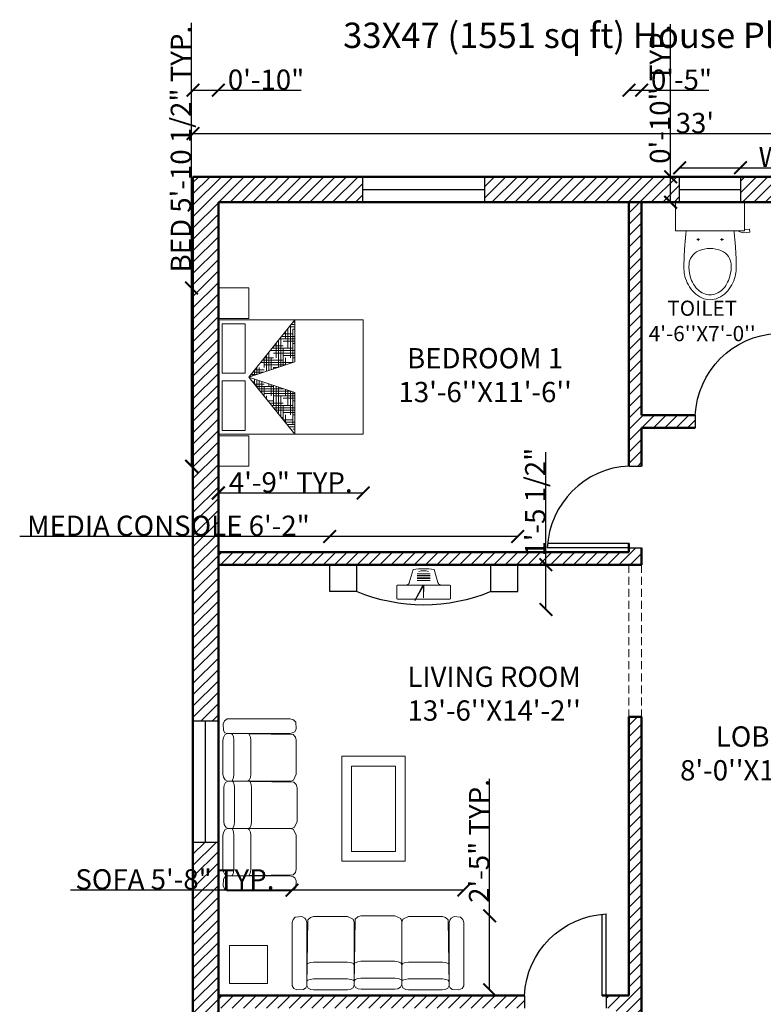
# Model space of a CAD drawing. Units: inches. Extents: x 1875 to 2385, y 1585 to 2263.
# Tile 2 of 3: x 1875 to 2168, y 1875 to 2263. Entities that reach past the tile are written whole.
import ezdxf

# ---------------------------------------------------------------- set-up
doc = ezdxf.new("R2010")
doc.units = ezdxf.units.IN
doc.header["$LTSCALE"] = 0.5
doc.linetypes.add('HIDDEN', pattern=[9.525, 6.35, -3.175])
for name, color, linetype, lineweight in [('A-ANNO-DIMS', 2, 'Continuous', 18), ('A-ANNO-TEXT', 7, 'Continuous', 25), ('A-AREA-IDEN', 7, 'Continuous', 25), ('A-FLOR-FIXT', 9, 'Continuous', 18), ('A-FURN', 8, 'Continuous', 18), ('A-WALL-HIDN', 56, 'HIDDEN', 18), ('A-WALL-PATT', 8, 'Continuous', 13), ('Doors', 42, 'Continuous', 25), ('Walls', 7, 'Continuous', 50), ('Windows', 140, 'Continuous', 25)]:
    doc.layers.add(name, color=color, linetype=linetype, lineweight=lineweight)
doc.layers.add('THIET-BI', color=21, linetype='Continuous')
doc.styles.get("Standard").update_dxf_attribs({"font": 'arial.ttf'})
doc.dimstyles.get("Standard").update_dxf_attribs({"dimtxt": 8, "dimasz": 5, "dimexe": 0.18, "dimexo": 0.0625, "dimgap": 0.09, "dimtad": 1, "dimdec": 1, "dimzin": 0, "dimdsep": 46, "dimlunit": 4, "dimtxsty": 'Standard', "dimblk": 'ARCHTICK', "dimcen": 0.09, "dimse1": 1, "dimse2": 1, "dimadec": 0, "dimazin": 0, "dimtfac": 1, "dimtdec": 1, "dimtofl": 0, "dimtmove": 0, "dimatfit": 3, "dimfxl": 1, "dimtolj": 1, "dimtzin": 0, "dimarcsym": 0})

# ---------------------------------------------------------------- blocks, each defined once
blk = doc.blocks.new('AP0B05')
for p, q in [((35, 100), (35, 880)), ((75, 100), (75, 878.9)), ((35, 100), (35, -20)), ((815, 100), (815, -20))]:
    blk.add_line(p, q)
blk.add_lwpolyline([(35, 100), (75, 100)])
blk.add_arc((-2.4, 62.6), 818.3, 2.62122, 87.37878)
blk = doc.blocks.new('12PCOU17')
at = {"color": 0, "linetype": 'ByBlock'}
for points in [[(-34.71, 34.72), (-33.66, 34.31), (-3.27, 34.3), (-1.81, 34.76), (-1.05, 35.2), (-0.38, 36.65), (-0.61, 39.84), (-1.73, 40.94), (-3.27, 41.4), (-33.66, 41.4), (-34.95, 40.5), (-35.65, 39.02), (-35.49, 35.83), (-34.71, 34.72)], [(-1.89, 11.91), (-1.66, 11.91), (-0.35, 14.68), (-0.35, 31.05), (-0.74, 32.58), (-1.89, 33.83), (-33.63, 34.3), (-34.84, 33.63), (-35.43, 32.38), (-35.68, 31), (-35.68, 14.74), (-35.43, 13.36), (-34.66, 11.99), (-33.44, 11.43), (-3, 11.44), (-1.66, 11.91)], [(-31.25, 11.43), (-31.06, 11.84), (-30.6, 13.09), (-30.4, 14.62), (-30.4, 31.12), (-30.6, 32.65), (-31.06, 33.9), (-31.81, 34.3)], [(-23.84, 11.43), (-22.99, 11.9), (-22.46, 13.15), (-22.23, 14.67), (-22.23, 31.07), (-22.46, 32.59), (-22.99, 33.84), (-23.12, 34.3)], [(-1.54, -10.96), (-1.31, -10.96), (0, -8.19), (0, 8.19), (-0.39, 9.71), (-1.54, 10.96), (-33.28, 11.44), (-34.5, 10.77), (-35.08, 9.51), (-35.33, 8.14), (-35.33, -8.13), (-35.08, -9.51), (-34.31, -10.87), (-33.1, -11.44), (-2.65, -11.43), (-1.31, -10.96)], [(-30.9, -11.44), (-30.72, -11.02), (-30.25, -9.77), (-30.05, -8.25), (-30.05, 8.26), (-30.25, 9.78), (-30.72, 11.03), (-31.47, 11.44)], [(-23.49, -11.44), (-22.64, -10.96), (-22.11, -9.72), (-21.88, -8.19), (-21.88, 8.2), (-22.11, 9.73), (-22.64, 10.97), (-22.77, 11.44)], [(-1.89, -11.91), (-1.66, -11.91), (-0.35, -14.68), (-0.35, -31.05), (-0.74, -32.58), (-1.89, -33.83), (-33.63, -34.3), (-34.84, -33.63), (-35.43, -32.38), (-35.68, -31), (-35.68, -14.74), (-35.43, -13.36), (-34.66, -11.99), (-33.44, -11.43), (-3, -11.44), (-1.66, -11.91)], [(-31.25, -11.43), (-31.06, -11.84), (-30.6, -13.09), (-30.4, -14.62), (-30.4, -31.12), (-30.6, -32.65), (-31.06, -33.9), (-31.81, -34.3)], [(-23.84, -11.43), (-22.99, -11.9), (-22.46, -13.15), (-22.23, -14.67), (-22.23, -31.07), (-22.46, -32.59), (-22.99, -33.84), (-23.12, -34.3)], [(-34.71, -34.72), (-33.66, -34.31), (-3.27, -34.3), (-1.81, -34.76), (-1.05, -35.2), (-0.38, -36.65), (-0.61, -39.84), (-1.73, -40.94), (-3.27, -41.4), (-33.66, -41.4), (-34.95, -40.5), (-35.65, -39.02), (-35.49, -35.83), (-34.71, -34.72)]]:
    blk.add_lwpolyline(points, dxfattribs=at)
blk = doc.blocks.new('*X4')
at = {"color": 0}
for p, q in [((20.174, 14.75), (20.277, 14.75)), ((20.188, 14.75), (20.188, 14.767)), ((20.199, 14.781), (20.277, 14.781)), ((20.25, 14.812), (20.277, 14.812)), ((20.25, 14.319), (20.25, 14.75)), ((20.062, 14.257), (20.062, 14.612)), ((20.094, 14.375), (20.094, 14.65)), ((20.098, 14.656), (20.125, 14.656)), ((20.124, 14.688), (20.25, 14.688)), ((20.125, 14.5), (20.125, 14.689)), ((20.149, 14.719), (20.277, 14.719)), ((20.156, 14.625), (20.156, 14.728)), ((20.219, 14.309), (20.219, 14.625)), ((20.25, 14.625), (20.277, 14.625)), ((19.973, 14.5), (20.25, 14.5)), ((19.998, 14.531), (20.277, 14.531)), ((20, 14.237), (20, 14.5)), ((20.023, 14.562), (20.277, 14.562)), ((20.031, 14.247), (20.031, 14.573)), ((20.125, 14.594), (20.277, 14.594)), ((20.188, 14.299), (20.188, 14.5)), ((19.875, 14.25), (19.875, 14.379)), ((19.875, 14.344), (20.277, 14.344)), ((19.906, 14.375), (19.906, 14.417)), ((19.922, 14.438), (20, 14.438)), ((19.948, 14.469), (20.125, 14.469)), ((19.969, 14.226), (19.969, 14.375)), ((20, 14.375), (20.277, 14.375)), ((20.125, 14.406), (20.277, 14.406)), ((20.156, 14.288), (20.156, 14.375)), ((20.25, 14.438), (20.277, 14.438)), ((19.746, 14.219), (19.875, 14.219)), ((19.75, 14.154), (19.75, 14.223)), ((19.772, 14.25), (20, 14.25)), ((19.781, 14.164), (19.781, 14.262)), ((19.797, 14.281), (20.125, 14.281)), ((19.812, 14.174), (19.812, 14.301)), ((19.822, 14.312), (20.229, 14.312)), ((19.844, 14.185), (19.844, 14.34)), ((19.938, 14.216), (19.938, 14.25)), ((19.702, 14.094), (19.779, 14.094)), ((19.719, 14.073), (19.719, 14.114)), ((19.721, 14.188), (19.75, 14.188)), ((19.75, 14.034), (19.75, 14.103)), ((19.781, 13.995), (19.781, 14.093)), ((19.727, 14.062), (19.873, 14.062)), ((19.752, 14.031), (19.875, 14.031)), ((19.812, 14), (19.812, 14.082)), ((19.875, 13.878), (19.875, 14)), ((19.875, 13.969), (20.156, 13.969)), ((19.906, 13.84), (19.906, 14.051)), ((19.938, 13.801), (19.938, 14.041)), ((19.969, 13.875), (19.969, 14.031)), ((20, 14), (20, 14.02)), ((20, 14), (20.061, 14)), ((20.062, 13.645), (20.062, 14)), ((20.094, 13.625), (20.094, 13.989)), ((20.125, 13.75), (20.125, 13.979)), ((20.156, 13.875), (20.156, 13.969)), ((19.827, 13.938), (20.25, 13.938)), ((19.853, 13.906), (20.125, 13.906)), ((19.878, 13.875), (20, 13.875)), ((20.031, 13.684), (20.031, 13.875)), ((20.125, 13.844), (20.277, 13.844)), ((20.219, 13.451), (20.219, 13.875)), ((20.25, 13.5), (20.25, 13.937)), ((20.25, 13.875), (20.277, 13.875)), ((19.953, 13.781), (20.277, 13.781)), ((19.978, 13.75), (20.25, 13.75)), ((20, 13.812), (20.277, 13.812)), ((20, 13.723), (20, 13.75)), ((20.003, 13.719), (20.125, 13.719)), ((20.188, 13.49), (20.188, 13.75)), ((20.079, 13.625), (20.277, 13.625)), ((20.104, 13.594), (20.277, 13.594)), ((20.125, 13.656), (20.277, 13.656)), ((20.156, 13.529), (20.156, 13.625)), ((20.25, 13.688), (20.277, 13.688)), ((20.129, 13.562), (20.25, 13.562)), ((20.205, 13.469), (20.277, 13.469)), ((20.25, 13.5), (20.277, 13.5)), ((20.23, 13.438), (20.277, 13.438)), ((20.255, 13.406), (20.277, 13.406))]:
    blk.add_line(p, q, dxfattribs=at)
blk = doc.blocks.new('MAT-P13')
for p, q in [((-1.17, 0), (-1.17, -0.4)), ((-1.17, 0), (-0.77, 0)), ((-0.77, 0), (-0.77, -0.4)), ((-0.75, 0), (0.75, 0)), ((-0.75, 0), (-0.75, -1.9)), ((0.75, 0), (0.75, -1.9)), ((0.77, 0), (1.17, 0)), ((0.77, 0), (0.77, -0.4)), ((1.17, 0), (1.17, -0.4)), ((-0.7, -0.05), (-0.7, -0.35)), ((-0.7, -0.05), (-0.05, -0.05)), ((-0.05, -0.35), (-0.05, -0.05)), ((0.05, -0.05), (0.7, -0.05)), ((0.05, -0.35), (0.05, -0.05)), ((0.7, -0.05), (0.7, -0.35)), ((-0.7, -0.35), (-0.05, -0.35)), ((0.05, -0.35), (0.7, -0.35)), ((-1.17, -0.4), (-0.77, -0.4)), ((-0.75, -1.003), (0, -0.4)), ((0, -0.4), (-0.75, -1.003)), ((0, -0.4), (-0.2, -1.003)), ((0, -0.4), (0.2, -1.003)), ((0, -0.4), (0.75, -1.003)), ((0.77, -0.4), (1.17, -0.4)), ((-0.75, -1.003), (-0.2, -1.003)), ((0.2, -1.003), (0.75, -1.003)), ((0.75, -1.9), (-0.75, -1.9))]:
    blk.add_line(p, q)
at = {"xscale": -1, "rotation": 90}
blk.add_blockref('*X4', (14.128, 19.274), dxfattribs=at)
blk = doc.blocks.new('toilet-1')
at = {"color": 0, "linetype": 'ByBlock'}
for p, q in [((-0.23, -0.02), (-0.23, -0.2116)), ((0.23, -0.02), (-0.23, -0.02)), ((0.23, -0.02), (0.23, -0.2116)), ((-0.23, -0.2116), (0.23, -0.2116)), ((-0.0793, -0.2587), (-0.0793, -0.2778)), ((0.0794, -0.2587), (0.0794, -0.2778)), ((0.1917, -0.2144), (0.2206, -0.225)), ((0.2206, -0.225), (0.266, -0.2187)), ((0.2633, -0.1997), (0.23, -0.2044)), ((0.266, -0.2187), (0.2633, -0.1997)), ((-0.0889, -0.2683), (-0.0697, -0.2683)), ((0.0889, -0.2683), (0.0698, -0.2683)), ((0, -0.6382), (0, -0.6382))]:
    blk.add_line(p, q, dxfattribs=at)
for centre, radius, start, end in [((3.5272, -0.6239), 3.7093, 173.69251, 175.15926), ((-3.527, -0.624), 3.7093, 4.84131, 6.31706), ((1.7368, -0.4519), 1.9109, 175.76982, 180.37578), ((-1.7366, -0.4519), 1.9109, 359.62422, 4.23018), ((-0.0408, -0.4398), 0.0996, 145.14967, 175.88096), ((-0.0312, -0.4465), 0.1114, 113.89968, 145.1485), ((0, -0.5169), 0.1884, 66.09393, 113.90607), ((0.0312, -0.4465), 0.1114, 34.8515, 66.10032), ((0.0409, -0.4398), 0.0996, 4.11904, 34.85033), ((0.0981, -0.4497), 0.2389, 175.88621, 195.59308), ((-0.098, -0.4497), 0.2389, 344.40692, 4.11379), ((0.0353, -0.463), 0.2093, 180.37466, 194.33753), ((0.055, -0.458), 0.2297, 194.33532, 209.62204), ((0.0961, -0.4503), 0.2369, 195.59686, 209.37705), ((-0.096, -0.4503), 0.2369, 330.62295, 344.40314), ((-0.0548, -0.458), 0.2297, 330.37879, 345.66551), ((-0.0351, -0.463), 0.2093, 345.6614, 359.62427), ((0.0647, -0.4524), 0.2409, 209.62726, 224.54888), ((0.0232, -0.4913), 0.1532, 209.38715, 226.54376), ((-0.0231, -0.4913), 0.1532, 313.45624, 330.61285), ((-0.0645, -0.4524), 0.2409, 315.45042, 330.37204), ((0.0178, -0.4986), 0.1751, 224.55199, 245.714), ((0.0152, -0.4997), 0.1416, 226.55015, 246.55272), ((0, -0.5347), 0.1034, 246.54933, 270.0042), ((0, -0.5347), 0.1034, 269.9958, 293.45067), ((-0.0151, -0.4997), 0.1416, 293.44728, 313.44985), ((-0.0176, -0.4986), 0.1751, 294.28649, 315.4485), ((0.0004, -0.538), 0.132, 245.58449, 269.87817), ((-0.0002, -0.538), 0.132, 270.12162, 294.4153)]:
    blk.add_arc(centre, radius, start, end, dxfattribs=at)
blk = doc.blocks.new('TVI01')
for p, q in [((-155, -10), (-213, -205)), ((-98, -73), (99, -73)), ((-98, -98), (99, -98)), ((-98, -123), (99, -123)), ((-98, -146), (99, -146)), ((155, -10), (214, -209)), ((-400, -254), (-400, -441)), ((-392, -244), (392, -244)), ((-98, -173), (99, -173)), ((-4, -248), (4, -432)), ((4, -248), (11, -244)), ((4, -248), (131, -471)), ((4, -248), (4, -432)), ((11, -244), (131, -471)), ((400, -254), (400, -441)), ((-392, -452), (392, -452))]:
    blk.add_line(p, q)
for centre, radius, start, end in [((0, -1208), 1208, 82.6216, 97.3784), ((0, -325), 295, 75.75, 104.25), ((-390, -254), 10, 100.3542, 183.7314), ((-75, -1338), 1112, 99.1976, 100.3542), ((-261, -191), 50, 279.1976, 343.4574), ((0, -248), 4, 0, 184.9692), ((261, -191), 50, 196.5426, 260.8024), ((75, -1338), 1112, 79.6458, 80.8024), ((390, -254), 10, 356.2686, 100.6983), ((-390, -442), 10, 176.2686, 259.6458), ((390, -442), 10, 280.3542, 3.7314)]:
    blk.add_arc(centre, radius, start, end)
blk = doc.blocks.new('A$C4C711776')
at = {"layer": 'THIET-BI'}
for p, q in [((180, 2160), (180, 2520)), ((180, 2520), (540, 2520)), ((540, 2160), (180, 2160)), ((180, 360), (180, 0)), ((180, 360), (540, 360)), ((180, 0), (540, 0))]:
    blk.add_line(p, q, dxfattribs=at)
at = {"layer": 'THIET-BI', "extrusion": (0, 0, -1)}
blk.add_ellipse((2340, 1260), major_axis=(1655, 1655), ratio=1, start_param=3.5322, end_param=4.321782, dxfattribs=at)
at = {"color": 0, "extrusion": (0, 0, -1), "xscale": 0.9000000000014551, "yscale": 0.9000000000014551, "zscale": -0.9, "rotation": 90}
blk.add_blockref('TVI01', (-485, 1261), dxfattribs=at)
blk = doc.blocks.new('_ArchTick')
at = {"color": 0, "linetype": 'ByBlock', "const_width": 0.15}
blk.add_lwpolyline([(-0.5, -0.5), (0.5, 0.5)], dxfattribs=at)
blk = doc.blocks.new('*D12')
at = {"layer": 'A-ANNO-DIMS', "color": 0, "lineweight": -2, "ltscale": 0.5, "transparency": 16777216}
blk.add_line((1943.28, 2218.51), (2339.28, 2218.51), dxfattribs=at)
at = {"layer": 'Defpoints', "color": 0, "ltscale": 0.5, "transparency": 16777216}
for p in [(2339.28, 2218.51), (1943.28, 2201.46), (2339.28, 2201.46)]:
    blk.add_point(p, dxfattribs=at)
at = {"layer": 'A-ANNO-DIMS', "color": 0, "lineweight": -2, "ltscale": 0.5, "transparency": 16777216, "xscale": 5, "yscale": 5, "zscale": 5, "rotation": 180}
blk.add_blockref('_ArchTick', (1943.28, 2218.51), dxfattribs=at)
at = {"layer": 'A-ANNO-DIMS', "color": 0, "lineweight": -2, "ltscale": 0.5, "transparency": 16777216, "xscale": 5, "yscale": 5, "zscale": 5}
blk.add_blockref('_ArchTick', (2339.28, 2218.51), dxfattribs=at)
at = {"layer": 'A-ANNO-DIMS', "color": 0, "ltscale": 0.5, "transparency": 16777216, "insert": (2141.28, 2222.69), "char_height": 8, "attachment_point": 5}
blk.add_mtext("\\A1;33'", dxfattribs=at)
blk = doc.blocks.new('WIN-48IN')
at = {"ltscale": 0.5}
blk.add_line((0, 0), (48, 0), dxfattribs=at)
blk.add_lwpolyline([(0, 5), (48, 5), (48, -5), (0, -5)], close=True, dxfattribs=at)
blk = doc.blocks.new('WIN-24IN')
at = {"ltscale": 0.5}
blk.add_line((0, 0), (24, 0), dxfattribs=at)
blk.add_lwpolyline([(0, 5), (24, 5), (24, -5), (0, -5)], close=True, dxfattribs=at)
blk = doc.blocks.new('*D24')
at = {"layer": 'A-ANNO-DIMS', "color": 0, "lineweight": -2, "ltscale": 0.5, "transparency": 16777216}
for p, q in [((1942.73, 2157.63), (1942.73, 2262.16)), ((1942.73, 2087.29), (1942.73, 2157.63))]:
    blk.add_line(p, q, dxfattribs=at)
at = {"layer": 'Defpoints', "color": 0, "ltscale": 0.5, "transparency": 16777216}
for p in [(1942.73, 2157.63), (1953.28, 2157.63), (1953.28, 2087.29)]:
    blk.add_point(p, dxfattribs=at)
at = {"layer": 'A-ANNO-DIMS', "color": 0, "lineweight": -2, "ltscale": 0.5, "transparency": 16777216, "xscale": 5, "yscale": 5, "zscale": 5}
for p, rotation in [((1942.73, 2157.63), 90), ((1942.73, 2087.29), 270)]:
    blk.add_blockref('_ArchTick', p, dxfattribs=dict(at, rotation=rotation))
at = {"layer": 'A-ANNO-DIMS', "color": 0, "ltscale": 0.5, "transparency": 16777216, "insert": (1938.51, 2212.39), "char_height": 8, "attachment_point": 5, "rotation": 90}
blk.add_mtext('\\A1;BED 5\'-10 1/2" TYP.', dxfattribs=at)
blk = doc.blocks.new('*D25')
at = {"layer": 'A-ANNO-DIMS', "color": 0, "lineweight": -2, "ltscale": 0.5, "transparency": 16777216}
blk.add_line((2010.4, 2076.74), (1953.28, 2076.74), dxfattribs=at)
at = {"layer": 'Defpoints', "color": 0, "ltscale": 0.5, "transparency": 16777216}
for p in [(1953.28, 2087.29), (2010.4, 2087.29), (1953.28, 2076.74)]:
    blk.add_point(p, dxfattribs=at)
at = {"layer": 'A-ANNO-DIMS', "color": 0, "lineweight": -2, "ltscale": 0.5, "transparency": 16777216, "xscale": 5, "yscale": 5, "zscale": 5, "rotation": 180}
blk.add_blockref('_ArchTick', (1953.28, 2076.74), dxfattribs=at)
at = {"layer": 'A-ANNO-DIMS', "color": 0, "lineweight": -2, "ltscale": 0.5, "transparency": 16777216, "xscale": 5, "yscale": 5, "zscale": 5}
blk.add_blockref('_ArchTick', (2010.4, 2076.74), dxfattribs=at)
at = {"layer": 'A-ANNO-DIMS', "color": 0, "ltscale": 0.5, "transparency": 16777216, "insert": (1981.84, 2080.91), "char_height": 8, "attachment_point": 5}
blk.add_mtext('\\A1;4\'-9" TYP.', dxfattribs=at)
blk = doc.blocks.new('*D26')
at = {"layer": 'A-ANNO-DIMS', "color": 0, "lineweight": -2, "ltscale": 0.5, "transparency": 16777216}
for p, q in [((2135.28, 2205.06), (2159.28, 2205.06)), ((2159.28, 2205.06), (2265.7, 2205.06))]:
    blk.add_line(p, q, dxfattribs=at)
at = {"layer": 'Defpoints', "color": 0, "ltscale": 0.5, "transparency": 16777216}
for p in [(2159.28, 2205.06), (2135.28, 2201.46), (2159.28, 2201.46)]:
    blk.add_point(p, dxfattribs=at)
at = {"layer": 'A-ANNO-DIMS', "color": 0, "lineweight": -2, "ltscale": 0.5, "transparency": 16777216, "xscale": 5, "yscale": 5, "zscale": 5, "rotation": 180}
blk.add_blockref('_ArchTick', (2135.28, 2205.06), dxfattribs=at)
at = {"layer": 'A-ANNO-DIMS', "color": 0, "lineweight": -2, "ltscale": 0.5, "transparency": 16777216, "xscale": 5, "yscale": 5, "zscale": 5}
blk.add_blockref('_ArchTick', (2159.28, 2205.06), dxfattribs=at)
at = {"layer": 'A-ANNO-DIMS', "color": 0, "ltscale": 0.5, "transparency": 16777216, "insert": (2214.99, 2209.29), "char_height": 8, "attachment_point": 5}
blk.add_mtext('\\A1;WINDOW 2\'-0" TYP.', dxfattribs=at)
blk = doc.blocks.new('*D27')
at = {"layer": 'A-ANNO-DIMS', "color": 0, "lineweight": -2, "ltscale": 0.5, "transparency": 16777216}
for p, q in [((2131.68, 2201.46), (2131.68, 2261.62)), ((2131.68, 2191.46), (2131.68, 2201.46))]:
    blk.add_line(p, q, dxfattribs=at)
at = {"layer": 'Defpoints', "color": 0, "ltscale": 0.5, "transparency": 16777216}
for p in [(2131.68, 2201.46), (2135.28, 2201.46), (2135.28, 2191.46)]:
    blk.add_point(p, dxfattribs=at)
at = {"layer": 'A-ANNO-DIMS', "color": 0, "lineweight": -2, "ltscale": 0.5, "transparency": 16777216, "xscale": 5, "yscale": 5, "zscale": 5}
for p, rotation in [((2131.68, 2201.46), 90), ((2131.68, 2191.46), 270)]:
    blk.add_blockref('_ArchTick', p, dxfattribs=dict(at, rotation=rotation))
at = {"layer": 'A-ANNO-DIMS', "color": 0, "ltscale": 0.5, "transparency": 16777216, "insert": (2127.51, 2234.04), "char_height": 8, "attachment_point": 5, "rotation": 90}
blk.add_mtext('\\A1;0\'-10" TYP.', dxfattribs=at)
blk = doc.blocks.new('*D28')
at = {"layer": 'A-ANNO-DIMS', "color": 0, "lineweight": -2, "ltscale": 0.5, "transparency": 16777216}
for p, q in [((1982.36, 1920.1), (1894.92, 1920.1)), ((2050.15, 1920.1), (1982.36, 1920.1))]:
    blk.add_line(p, q, dxfattribs=at)
at = {"layer": 'Defpoints', "color": 0, "ltscale": 0.5, "transparency": 16777216}
for p in [(1982.36, 1920.1), (1982.36, 1909.93), (2050.15, 1909.93)]:
    blk.add_point(p, dxfattribs=at)
at = {"layer": 'A-ANNO-DIMS', "color": 0, "lineweight": -2, "ltscale": 0.5, "transparency": 16777216, "xscale": 5, "yscale": 5, "zscale": 5, "rotation": 180}
blk.add_blockref('_ArchTick', (1982.36, 1920.1), dxfattribs=at)
at = {"layer": 'A-ANNO-DIMS', "color": 0, "lineweight": -2, "ltscale": 0.5, "transparency": 16777216, "xscale": 5, "yscale": 5, "zscale": 5}
blk.add_blockref('_ArchTick', (2050.15, 1920.1), dxfattribs=at)
at = {"layer": 'A-ANNO-DIMS', "color": 0, "ltscale": 0.5, "transparency": 16777216, "insert": (1936.14, 1924.33), "char_height": 8, "attachment_point": 5}
blk.add_mtext('\\A1;SOFA 5\'-8" TYP.', dxfattribs=at)
blk = doc.blocks.new('*D29')
at = {"layer": 'A-ANNO-DIMS', "color": 0, "lineweight": -2, "ltscale": 0.5, "transparency": 16777216}
for p, q in [((2060.32, 1909.93), (2060.32, 1964.01)), ((2060.32, 1880.72), (2060.32, 1909.93))]:
    blk.add_line(p, q, dxfattribs=at)
at = {"layer": 'Defpoints', "color": 0, "ltscale": 0.5, "transparency": 16777216}
for p in [(2050.15, 1909.93), (2060.32, 1909.93), (2050.15, 1880.72)]:
    blk.add_point(p, dxfattribs=at)
at = {"layer": 'A-ANNO-DIMS', "color": 0, "lineweight": -2, "ltscale": 0.5, "transparency": 16777216, "xscale": 5, "yscale": 5, "zscale": 5}
for p, rotation in [((2060.32, 1909.93), 90), ((2060.32, 1880.72), 270)]:
    blk.add_blockref('_ArchTick', p, dxfattribs=dict(at, rotation=rotation))
at = {"layer": 'A-ANNO-DIMS', "color": 0, "ltscale": 0.5, "transparency": 16777216, "insert": (2056.15, 1939.47), "char_height": 8, "attachment_point": 5, "rotation": 90}
blk.add_mtext('\\A1;2\'-5" TYP.', dxfattribs=at)
blk = doc.blocks.new('*D36')
at = {"layer": 'A-ANNO-DIMS', "color": 0, "lineweight": -2, "ltscale": 0.5, "transparency": 16777216}
for p, q in [((1997.24, 2059.58), (1874.91, 2059.58)), ((2071.4, 2059.58), (1997.24, 2059.58))]:
    blk.add_line(p, q, dxfattribs=at)
at = {"layer": 'Defpoints', "color": 0, "ltscale": 0.5, "transparency": 16777216}
for p in [(1997.24, 2059.58), (1997.24, 2048.46), (2071.4, 2048.46)]:
    blk.add_point(p, dxfattribs=at)
at = {"layer": 'A-ANNO-DIMS', "color": 0, "lineweight": -2, "ltscale": 0.5, "transparency": 16777216, "xscale": 5, "yscale": 5, "zscale": 5, "rotation": 180}
blk.add_blockref('_ArchTick', (1997.24, 2059.58), dxfattribs=at)
at = {"layer": 'A-ANNO-DIMS', "color": 0, "lineweight": -2, "ltscale": 0.5, "transparency": 16777216, "xscale": 5, "yscale": 5, "zscale": 5}
blk.add_blockref('_ArchTick', (2071.4, 2059.58), dxfattribs=at)
at = {"layer": 'A-ANNO-DIMS', "color": 0, "ltscale": 0.5, "transparency": 16777216, "insert": (1933.58, 2063.81), "char_height": 8, "attachment_point": 5}
blk.add_mtext('\\A1;MEDIA CONSOLE 6\'-2"', dxfattribs=at)
blk = doc.blocks.new('*D37')
at = {"layer": 'A-ANNO-DIMS', "color": 0, "lineweight": -2, "ltscale": 0.5, "transparency": 16777216}
for p, q in [((2082.52, 2048.46), (2082.52, 2092.79)), ((2082.52, 2030.8), (2082.52, 2048.46))]:
    blk.add_line(p, q, dxfattribs=at)
at = {"layer": 'Defpoints', "color": 0, "ltscale": 0.5, "transparency": 16777216}
for p in [(2071.4, 2048.46), (2082.52, 2048.46), (2071.4, 2030.8)]:
    blk.add_point(p, dxfattribs=at)
at = {"layer": 'A-ANNO-DIMS', "color": 0, "lineweight": -2, "ltscale": 0.5, "transparency": 16777216, "xscale": 5, "yscale": 5, "zscale": 5}
for p, rotation in [((2082.52, 2048.46), 90), ((2082.52, 2030.8), 270)]:
    blk.add_blockref('_ArchTick', p, dxfattribs=dict(at, rotation=rotation))
at = {"layer": 'A-ANNO-DIMS', "color": 0, "ltscale": 0.5, "transparency": 16777216, "insert": (2078.3, 2073.13), "char_height": 8, "attachment_point": 5, "rotation": 90}
blk.add_mtext('\\A1;1\'-5 1/2"', dxfattribs=at)
blk = doc.blocks.new('*D40')
at = {"layer": 'A-ANNO-DIMS', "color": 0, "lineweight": -2, "ltscale": 0.5, "transparency": 16777216}
for p, q in [((1943.28, 2235.61), (1953.28, 2235.61)), ((1953.28, 2235.61), (1985.95, 2235.61))]:
    blk.add_line(p, q, dxfattribs=at)
at = {"layer": 'Defpoints', "color": 0, "ltscale": 0.5, "transparency": 16777216}
for p in [(1953.28, 2235.61), (1943.28, 2201.46), (1953.28, 2191.46)]:
    blk.add_point(p, dxfattribs=at)
at = {"layer": 'A-ANNO-DIMS', "color": 0, "lineweight": -2, "ltscale": 0.5, "transparency": 16777216, "xscale": 5, "yscale": 5, "zscale": 5, "rotation": 180}
blk.add_blockref('_ArchTick', (1943.28, 2235.61), dxfattribs=at)
at = {"layer": 'A-ANNO-DIMS', "color": 0, "lineweight": -2, "ltscale": 0.5, "transparency": 16777216, "xscale": 5, "yscale": 5, "zscale": 5}
blk.add_blockref('_ArchTick', (1953.28, 2235.61), dxfattribs=at)
at = {"layer": 'A-ANNO-DIMS', "color": 0, "ltscale": 0.5, "transparency": 16777216, "insert": (1972.11, 2239.78), "char_height": 8, "attachment_point": 5}
blk.add_mtext('\\A1;0\'-10"', dxfattribs=at)
blk = doc.blocks.new('*D41')
at = {"layer": 'A-ANNO-DIMS', "color": 0, "lineweight": -2, "ltscale": 0.5, "transparency": 16777216}
for p, q in [((2115.28, 2235.61), (2120.28, 2235.61)), ((2120.28, 2235.61), (2146.73, 2235.61))]:
    blk.add_line(p, q, dxfattribs=at)
at = {"layer": 'Defpoints', "color": 0, "ltscale": 0.5, "transparency": 16777216}
for p in [(2120.28, 2235.61), (2115.28, 2191.46), (2120.28, 2191.46)]:
    blk.add_point(p, dxfattribs=at)
at = {"layer": 'A-ANNO-DIMS', "color": 0, "lineweight": -2, "ltscale": 0.5, "transparency": 16777216, "xscale": 5, "yscale": 5, "zscale": 5, "rotation": 180}
blk.add_blockref('_ArchTick', (2115.28, 2235.61), dxfattribs=at)
at = {"layer": 'A-ANNO-DIMS', "color": 0, "lineweight": -2, "ltscale": 0.5, "transparency": 16777216, "xscale": 5, "yscale": 5, "zscale": 5}
blk.add_blockref('_ArchTick', (2120.28, 2235.61), dxfattribs=at)
at = {"layer": 'A-ANNO-DIMS', "color": 0, "ltscale": 0.5, "transparency": 16777216, "insert": (2136.01, 2239.78), "char_height": 8, "attachment_point": 5}
blk.add_mtext('\\A1;0\'-5"', dxfattribs=at)

msp = doc.modelspace()

# ---------------------------------------------------------------- hatches: boundary and pattern name
at = {"layer": 'A-WALL-PATT', "ltscale": 0.5, "transparency": 33554585}
h = msp.add_hatch(dxfattribs=at)
h.set_pattern_fill('ANSI31', color=256)
h.paths.add_polyline_path([(2010.28, 2201.46), (1943.28, 2201.46), (1943.28, 1986.92), (1953.28, 1986.92), (1953.28, 2191.46), (2010.28, 2191.46)])
h.paths.add_polyline_path([(2135.28, 2201.46), (2058.28, 2201.46), (2058.28, 2191.46), (2135.28, 2191.46)])
h.paths.add_polyline_path([(2120.28, 2191.46), (2115.28, 2191.46), (2115.28, 2087.38), (2120.28, 2087.38), (2120.28, 2102.46), (2141.45, 2102.46), (2141.45, 2107.46), (2120.28, 2107.46)])
h.paths.add_polyline_path([(2230.28, 2201.46), (2159.28, 2201.46), (2159.28, 2191.46), (2160.9, 2191.46), (2230.28, 2191.46)])
h.paths.add_polyline_path([(2179.28, 2191.46), (2174.28, 2191.46), (2174.28, 2107.46), (2173.71, 2107.46), (2173.71, 2107.42), (2173.71, 2102.46), (2174.28, 2102.46), (2174.28, 2087.38), (2179.28, 2087.38)])
h.paths.add_polyline_path([(2339.28, 2201.46), (2278.28, 2201.46), (2278.28, 2191.46), (2329.28, 2191.46), (2329.28, 2033.69), (2339.28, 2033.69)])
h.paths.add_polyline_path([(2329.28, 2053.46), (2179.28, 2053.46), (2179.28, 2055.12), (2179.25, 2055.12), (2174.28, 2055.12), (2174.28, 2048.46), (2216.28, 2048.46), (2216.28, 2027.77), (2221.28, 2027.77), (2221.28, 2048.46), (2329.28, 2048.46)])
h = msp.add_hatch(dxfattribs=at)
h.set_pattern_fill('ANSI31', color=256)
h.paths.add_polyline_path([(2120.28, 2055.12), (2115.28, 2055.12), (2115.28, 2053.46), (1953.28, 2053.46), (1953.28, 2048.46), (2120.28, 2048.46)])
h.paths.add_polyline_path([(2339.28, 2009.69), (2329.28, 2009.69), (2329.28, 1958.74), (2339.28, 1958.74)])
h.paths.add_polyline_path([(2140.01, 1729.46), (2138.58, 1729.46), (2120.28, 1729.46), (2120.28, 1988.46), (2115.28, 1988.46), (2115.28, 1878.46), (2106.32, 1878.46), (2106.32, 1878.42), (2106.32, 1873.46), (2110.28, 1873.46), (2110.28, 1719.46), (2140.01, 1719.46)])
h.paths.add_polyline_path([(2074.06, 1878.46), (1953.28, 1878.46), (1953.28, 1873.46), (2074.06, 1873.46)])
h.paths.add_polyline_path([(1953.28, 1938.92), (1943.28, 1938.92), (1943.28, 1637.46), (1953.28, 1637.46), (1953.28, 1647.46)])
h.paths.add_polyline_path([(2329.28, 1729.46), (2164.01, 1729.46), (2164.01, 1719.46), (2329.28, 1719.46)])
h.paths.add_polyline_path([(2185.28, 1837.05), (2180.28, 1837.05), (2180.28, 1818.46), (2158.46, 1818.46), (2158.46, 1813.46), (2180.28, 1813.46), (2180.28, 1729.46), (2185.28, 1729.46)])
h.paths.add_polyline_path([(2126.2, 1818.46), (2120.28, 1818.46), (2120.28, 1813.46), (2126.2, 1813.46), (2126.2, 1813.5)], flags=17)
h.paths.add_polyline_path([(2339.28, 1910.74), (2329.28, 1910.74), (2329.28, 1823.21), (2339.28, 1823.21)])
h.paths.add_polyline_path([(2339.28, 1775.21), (2329.28, 1775.21), (2329.28, 1701.57), (2339.28, 1701.57)])
h.paths.add_polyline_path([(2339.28, 1665.57), (2329.28, 1665.57), (2329.28, 1647.46), (2110.28, 1647.46), (2102.69, 1647.46), (2102.69, 1637.46), (2110.28, 1637.46), (2339.28, 1637.46)])

# ---------------------------------------------------------------- linework, layer by layer
at = {"layer": 'A-FURN', "ltscale": 0.5}
for points in [[(2001.99, 1972.87), (2027.04, 1972.87), (2027.04, 1931.51), (2001.99, 1931.51)], [(2005.81, 1969.04), (2023.22, 1969.04), (2023.22, 1935.33), (2005.81, 1935.33)], [(1957.62, 1898.24), (1972.64, 1898.24), (1972.64, 1883.24), (1957.62, 1883.24)]]:
    msp.add_lwpolyline(points, close=True, dxfattribs=at)
at = {"layer": 'A-WALL-HIDN'}
for p, q in [((2115.28, 2048.46), (2115.28, 1988.46)), ((2120.28, 2048.46), (2120.28, 1988.46))]:
    msp.add_line(p, q, dxfattribs=at)
at = {"layer": 'Walls'}
for p, q in [((1943.28, 2201.46), (2339.28, 2201.46)), ((1943.28, 2201.46), (1943.28, 1637.46)), ((1953.28, 2191.46), (2329.28, 2191.46)), ((1953.28, 2191.46), (1953.28, 1637.46)), ((2115.28, 2191.46), (2115.28, 2087.38)), ((2120.28, 2191.46), (2120.28, 2107.46)), ((2120.28, 2107.46), (2141.45, 2107.46)), ((2120.28, 2102.46), (2141.45, 2102.46)), ((2120.28, 2102.46), (2120.28, 2087.38)), ((2115.28, 2056.77), (2115.28, 2053.46)), ((1953.28, 2053.46), (2115.28, 2053.46)), ((1953.28, 2048.46), (2120.28, 2048.46)), ((2115.28, 1988.46), (2115.28, 1878.46)), ((2120.28, 1988.46), (2120.28, 1729.46)), ((1953.28, 1878.46), (2074.06, 1878.46)), ((2104.66, 1878.46), (2115.28, 1878.46))]:
    msp.add_line(p, q, dxfattribs=at)
at = {"layer": 'Walls', "ltscale": 0.5}
for p, q in [((2120.28, 2048.46), (2120.28, 2055.12)), ((2115.28, 1988.46), (2120.28, 1988.46))]:
    msp.add_line(p, q, dxfattribs=at)

# ---------------------------------------------------------------- block references
at = {"layer": 'A-FLOR-FIXT', "ltscale": 0.5, "xscale": 59.18137808131736, "yscale": 59.18137808131736, "zscale": 59.18137808131736}
msp.add_blockref('toilet-1', (2147.28, 2192.64), dxfattribs=at)
at = {"layer": 'A-FURN', "ltscale": 0.5, "rotation": 90}
for name, p, xscale, yscale, zscale in [('MAT-P13', (1953.28, 2122.46), 30.05916968857566, 30.05916968857566, 30.05916968857566), ('12PCOU17', (2016.26, 1909.93), 0.8187222260571754, 0.8187222260571754, 0.8187222260571754)]:
    msp.add_blockref(name, p, dxfattribs=dict(at, xscale=xscale, yscale=yscale, zscale=zscale))
at = {"layer": 'A-FURN', "xscale": 0.0294268908759337, "yscale": 0.0294268908759337, "zscale": 0.0294268908759337, "rotation": 90}
msp.add_blockref('A$C4C711776', (2071.4, 2032.57), dxfattribs=at)
at = {"layer": 'A-FURN', "ltscale": 0.5, "xscale": 0.8187222260571754, "yscale": 0.8187222260571754, "zscale": 0.8187222260571754}
msp.add_blockref('12PCOU17', (1984.32, 1953.76), dxfattribs=at)
at = {"layer": 'Doors', "xscale": -0.0413587909994788, "yscale": 0.0413587909994788, "zscale": 0.0413587909994788}
for p in [(2175.15, 2103.29), (2107.76, 1874.29)]:
    msp.add_blockref('AP0B05', p, dxfattribs=at)
at = {"layer": 'Doors', "xscale": 0.0413587909994788, "yscale": 0.0413587909994788, "zscale": 0.0413587909994788, "rotation": 90.0000000000009}
msp.add_blockref('AP0B05', (2119.46, 2053.67), dxfattribs=at)
at = {"layer": 'Windows'}
for name, p in [('WIN-48IN', (2010.28, 2196.46)), ('WIN-24IN', (2135.28, 2196.46))]:
    msp.add_blockref(name, p, dxfattribs=at)
at = {"layer": 'Windows', "rotation": 89.99999999999837}
msp.add_blockref('WIN-48IN', (1948.28, 1938.92), dxfattribs=at)

# ---------------------------------------------------------------- texts
at = {"layer": 'A-ANNO-TEXT', "ltscale": 0.5}
msp.add_text('33X47 (1551 sq ft) House Plan - South Face', height=10, dxfattribs=at).set_placement((2002.52, 2252.29))
at = {"layer": 'A-AREA-IDEN', "ltscale": 0.5, "attachment_point": 1}
for s, insert, char_height in [("\\pxqc;TOILET\\P4'-6''X7'-0''", (2106.99, 2152.63), 6), ("\\pxqc;BEDROOM 1\\P13'-6''X11'-6''", (2021.34, 2133.91), 8), ("\\pxqc;LIVING ROOM\\P13'-6''X14'-2''", (2024.91, 2008.26), 8), ("\\pxqc;LOBBY\\P8'-0''X14'-2''", (2129.42, 1984.69), 8)]:
    msp.add_mtext_dynamic_manual_height_columns(s, width=74.3766, gutter_width=12.5, heights=[0], dxfattribs=dict(at, insert=insert, char_height=char_height))

# ---------------------------------------------------------------- dimensions: what is measured, and where the dimension line sits
at = {"layer": 'A-ANNO-DIMS', "ltscale": 0.5}
for base, p1, p2, angle, text, picture, middle in [((1942.73, 2157.63), (1953.28, 2087.29), (1953.28, 2157.63), 90, 'BED <> TYP.', '*D24', (1938.51, 2212.39)), ((2131.68, 2201.46), (2135.28, 2191.46), (2135.28, 2201.46), 90, '<> TYP.', '*D27', (2127.51, 2234.04)), ((1953.28, 2076.74), (2010.4, 2087.29), (1953.28, 2087.29), 180, '<> TYP.', '*D25', (1981.84, 2080.91)), ((1997.24, 2059.58), (2071.4, 2048.46), (1997.24, 2048.46), 180, 'MEDIA CONSOLE <>', '*D36', (1933.58, 2063.81)), ((2060.32, 1909.93), (2050.15, 1880.72), (2050.15, 1909.93), 90, '<> TYP.', '*D29', (2056.15, 1939.47)), ((1982.36, 1920.1), (2050.15, 1909.93), (1982.36, 1909.93), 180, 'SOFA <> TYP.', '*D28', (1936.14, 1924.33))]:
    dim = msp.add_linear_dim(base=base, p1=p1, p2=p2, angle=angle, text=text, dimstyle='Standard', override={"dimdec": 1, "dimlfac": 1, "dimrnd": 0, "dimzin": 1, "dimdsep": 46, "dimlunit": 4, "dimfrac": 2}, dxfattribs=at)
    dim.commit()
    dim.dimension.update_dxf_attribs({"geometry": picture, "text_midpoint": middle})
for base, p1, p2, override, picture, middle in [((1953.28, 2235.61), (1943.28, 2201.46), (1953.28, 2191.46), {"dimdec": 1, "dimlfac": 1, "dimrnd": 0, "dimzin": 1, "dimdsep": 46, "dimlunit": 4, "dimfrac": 2}, '*D40', (1972.11, 2239.78)), ((2120.28, 2235.61), (2115.28, 2191.46), (2120.28, 2191.46), {"dimdec": 1, "dimlfac": 1, "dimrnd": 0, "dimzin": 1, "dimdsep": 46, "dimlunit": 4, "dimfrac": 2}, '*D41', (2136.01, 2239.78)), ((2339.28, 2218.51), (1943.28, 2201.46), (2339.28, 2201.46), {"dimclrd": 0, "dimclre": 0, "dimclrt": 0}, '*D12', (2141.28, 2222.69))]:
    dim = msp.add_linear_dim(base=base, p1=p1, p2=p2, dimstyle='Standard', override=override, dxfattribs=at)
    dim.commit()
    dim.dimension.update_dxf_attribs({"geometry": picture, "text_midpoint": middle})
dim = msp.add_linear_dim(base=(2159.28, 2205.06), p1=(2135.28, 2201.46), p2=(2159.28, 2201.46), text='WINDOW <> TYP.', dimstyle='Standard', override={"dimdec": 1, "dimlfac": 1, "dimrnd": 0, "dimzin": 1, "dimdsep": 46, "dimlunit": 4, "dimfrac": 2}, dxfattribs=at)
dim.commit()
dim.dimension.update_dxf_attribs({"geometry": '*D26', "text_midpoint": (2214.99, 2209.29)})
dim = msp.add_linear_dim(base=(2082.52, 2048.46), p1=(2071.4, 2030.8), p2=(2071.4, 2048.46), angle=90, dimstyle='Standard', override={"dimdec": 1, "dimlfac": 1, "dimrnd": 0, "dimzin": 1, "dimdsep": 46, "dimlunit": 4, "dimfrac": 2}, dxfattribs=at)
dim.commit()
dim.dimension.update_dxf_attribs({"geometry": '*D37', "text_midpoint": (2078.3, 2073.13)})

doc.saveas('drawing.dxf')
